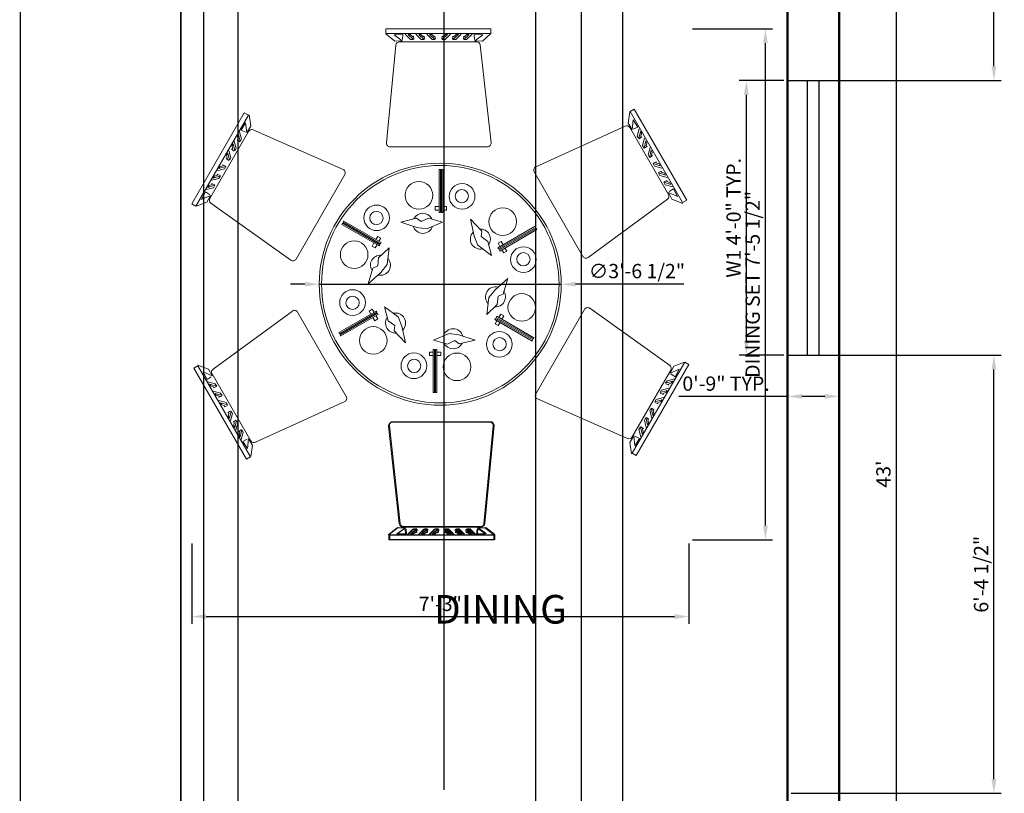
# Model space of a CAD drawing. Units: inches. Extents: x 1905 to 2315, y 3232 to 3824.
# Tile 5 of 8: x 2143 to 2315, y 3479 to 3615. Entities that reach past the tile are written whole.
import ezdxf

# ---------------------------------------------------------------- set-up
doc = ezdxf.new("R2010")
doc.units = ezdxf.units.IN
for name, color, linetype, lineweight in [('A-ANNO-DIMS', 2, 'Continuous', 18), ('A-AREA-IDEN', 7, 'Continuous', 25), ('A-FURN', 8, 'Continuous', 18), ('wall', 2, 'Continuous', 50), ('WINDOW', 60, 'Continuous', 25)]:
    doc.layers.add(name, color=color, linetype=linetype, lineweight=lineweight)
doc.styles.get("Standard").update_dxf_attribs({"font": 'arial.ttf'})
doc.dimstyles.new('ISO-25', dxfattribs={"dimtxt": 2.5, "dimasz": 2.5, "dimexe": 1.25, "dimexo": 0.625, "dimtad": 1, "dimdec": 1, "dimlunit": 3, "dimtxsty": 'Standard', "dimcen": 2.5, "dimadec": 0, "dimazin": 0, "dimtfac": 1, "dimtdec": 1, "dimtmove": 0, "dimatfit": 3, "dimfxl": 1, "dimarcsym": 0})

# ---------------------------------------------------------------- blocks, each defined once
blk = doc.blocks.new('A$C45501D90')
for p, q in [((-242.2, 1133.5), (224, 1133.5)), ((-242.2, 1112.8), (-242.2, 1133.5)), ((224, 1112.8), (-242.2, 1112.8)), ((-242.2, 1111.2), (-202.3, 1079.2)), ((-203.9, 1106.4), (-165.6, 1108)), ((-168.8, 1080.8), (-203.9, 1106.4)), ((-165.6, 1108), (-167.2, 1085.6)), ((-156, 1109.6), (-132, 1085.6)), ((-119.3, 1085.6), (-143.2, 1108)), ((-143.2, 1108), (-133.6, 1108)), ((-133.6, 1108), (-122.5, 1098.4)), ((-122.5, 1098.4), (-119.3, 1101.6)), ((-119.3, 1101.6), (-117.7, 1087.2)), ((-108.1, 1109.6), (-84.1, 1085.6)), ((-71.4, 1085.6), (-95.3, 1108)), ((-95.3, 1108), (-85.7, 1108)), ((-85.7, 1108), (-74.6, 1098.4)), ((-74.6, 1098.4), (-71.4, 1101.6)), ((-71.4, 1101.6), (-69.8, 1087.2)), ((-60.2, 1109.6), (-36.2, 1085.6)), ((-23.5, 1085.6), (-47.4, 1108)), ((-47.4, 1108), (-37.8, 1108)), ((-37.8, 1108), (-26.7, 1098.4)), ((-26.7, 1098.4), (-23.5, 1101.6)), ((-23.5, 1101.6), (-21.9, 1087.2)), ((8.5, 1101.6), (6.9, 1087.2)), ((8.5, 1085.6), (32.4, 1108)), ((11.6, 1098.4), (8.5, 1101.6)), ((22.8, 1108), (11.6, 1098.4)), ((45.2, 1109.6), (21.2, 1085.6)), ((32.4, 1108), (22.8, 1108)), ((56.3, 1101.6), (54.8, 1087.2)), ((56.3, 1085.6), (80.3, 1108)), ((59.5, 1098.4), (56.3, 1101.6)), ((70.7, 1108), (59.5, 1098.4)), ((93.1, 1109.6), (69.1, 1085.6)), ((80.3, 1108), (70.7, 1108)), ((104.2, 1101.6), (102.6, 1087.2)), ((104.2, 1085.6), (128.2, 1108)), ((107.4, 1098.4), (104.2, 1101.6)), ((118.6, 1108), (107.4, 1098.4)), ((141, 1109.6), (117, 1085.6)), ((128.2, 1108), (118.6, 1108)), ((188.9, 1106.4), (150.5, 1108)), ((150.5, 1108), (152.1, 1085.6)), ((153.7, 1080.8), (188.9, 1106.4)), ((224, 1112.8), (187.3, 1079.2)), ((224, 1133.5), (224, 1112.8)), ((-197.3, 1061.6), (-238.9, 627.6)), ((-202.3, 1079.2), (-168.8, 1080.8)), ((161.8, 1076.1), (-181.4, 1076.1)), ((-132, 1085.6), (-119.3, 1085.6)), ((-84.1, 1085.6), (-71.4, 1085.6)), ((-36.2, 1085.6), (-23.5, 1085.6)), ((21.2, 1085.6), (8.5, 1085.6)), ((69.1, 1085.6), (56.3, 1085.6)), ((117, 1085.6), (104.2, 1085.6)), ((187.3, 1079.2), (153.7, 1080.8)), ((225.2, 627.8), (177.6, 1061.8)), ((-1102.7, 357), (-869.7, 760.7)), ((-851.7, 750.4), (-1084.8, 346.6)), ((-869.7, 760.7), (-851.7, 750.4)), ((-848.7, 752.3), (-841, 701.8)), ((841.2, 765.3), (833.5, 714.8)), ((842.6, 766.1), (860.5, 776.5)), ((1075.7, 362.4), (842.6, 766.1)), ((860.5, 776.5), (1093.6, 372.8)), ((-863.7, 716.7), (-884.3, 684.4)), ((-859.2, 673.6), (-863.7, 716.7)), ((-841, 701.8), (-859.2, 673.6)), ((820.7, 701.7), (424.1, 520.7)), ((833.5, 714.8), (851.7, 686.6)), ((851.7, 686.6), (856.2, 729.8)), ((856.2, 729.8), (876.7, 697.4)), ((-851, 678.1), (-1022.6, 380.9)), ((-895.4, 665), (-900.2, 656.7)), ((-900.2, 656.7), (-897.5, 642.2)), ((-888.1, 633.1), (-895.4, 665)), ((-890.4, 676.9), (-881.7, 644.2)), ((-884.3, 684.4), (-864.1, 674.6)), ((-431.1, 509), (-830.8, 684.8)), ((1012.8, 397.9), (841.2, 695.1)), ((876.7, 697.4), (856.6, 687.6)), ((882.9, 689.9), (874.2, 657.2)), ((874.2, 657.2), (880.6, 646.1)), ((880.6, 646.1), (887.9, 678)), ((887.9, 678), (892.7, 669.7)), ((892.7, 669.7), (890, 655.2)), ((-919.4, 623.5), (-924.2, 615.2)), ((-924.2, 615.2), (-921.5, 600.8)), ((-912, 591.6), (-919.4, 623.5)), ((-914.4, 635.4), (-905.6, 602.7)), ((-897.5, 642.2), (-901.9, 641.1)), ((-901.9, 641.1), (-890.2, 632.5)), ((-881.7, 644.2), (-888.1, 633.1)), ((894.4, 654.1), (882.7, 645.5)), ((890, 655.2), (894.4, 654.1)), ((906.9, 648.4), (898.1, 615.7)), ((898.1, 615.7), (904.5, 604.6)), ((904.5, 604.6), (911.9, 636.5)), ((918.3, 612.6), (906.7, 604)), ((911.9, 636.5), (916.7, 628.2)), ((916.7, 628.2), (914, 613.8)), ((914, 613.8), (918.3, 612.6)), ((-943.3, 582), (-948.1, 573.8)), ((-948.1, 573.8), (-945.4, 559.3)), ((-936, 550.1), (-943.3, 582)), ((-938.3, 593.9), (-929.6, 561.2)), ((-921.5, 600.8), (-925.8, 599.6)), ((-925.8, 599.6), (-914.2, 591)), ((-905.6, 602.7), (-912, 591.6)), ((-223, 610.1), (209.4, 610.1)), ((930.8, 606.9), (922.1, 574.2)), ((922.1, 574.2), (928.4, 563.1)), ((928.4, 563.1), (935.8, 595.1)), ((942.3, 571.1), (930.6, 562.6)), ((935.8, 595.1), (940.6, 586.8)), ((940.6, 586.8), (937.9, 572.3)), ((937.9, 572.3), (942.3, 571.1)), ((-978.5, 521.2), (-964.6, 526.1)), ((-964.6, 526.1), (-965.7, 530.5)), ((-965.7, 530.5), (-952.5, 524.7)), ((-945.4, 559.3), (-949.8, 558.1)), ((-949.8, 558.1), (-938.1, 549.6)), ((-929.6, 561.2), (-936, 550.1)), ((950.8, 524.4), (944.4, 535.5)), ((944.4, 535.5), (975.7, 525.9)), ((958.2, 543.5), (945, 537.7)), ((983.5, 515.7), (950.8, 524.4)), ((957.1, 539.1), (958.2, 543.5)), ((970.9, 534.2), (957.1, 539.1)), ((975.7, 525.9), (970.9, 534.2)), ((-975.9, 481), (-1007.2, 471.4)), ((-1002.4, 479.7), (-988.5, 484.6)), ((-991, 502.7), (-958.3, 511.4)), ((-988.5, 484.6), (-989.7, 489)), ((-989.7, 489), (-976.5, 483.2)), ((-951.9, 522.5), (-983.2, 512.9)), ((-983.2, 512.9), (-978.5, 521.2)), ((-982.3, 469.9), (-975.9, 481)), ((-958.3, 511.4), (-951.9, 522.5)), ((-639.9, 111.9), (-423.7, 486.4)), ((-5.6, 508.7, 90.8), (0.4, 508.7, 90.8)), ((-5.6, 317.7, 90.8), (-5.6, 508.7, 90.8)), ((0.4, 508.7, 90.8), (0.4, 317.7, 90.8)), ((5.8, 317.7, 90.8), (5.8, 508.7, 90.8)), ((5.8, 508.7, 90.8), (11.8, 508.7, 90.8)), ((11.8, 508.7, 90.8), (11.8, 317.7, 90.8)), ((416.9, 498.2), (633.1, 123.7)), ((968.4, 494), (999.7, 484.4)), ((974.7, 483), (968.4, 494)), ((982.2, 502), (968.9, 496.2)), ((1007.4, 474.2), (974.7, 483)), ((981, 497.6), (982.2, 502)), ((994.9, 492.7), (981, 497.6)), ((999.7, 484.4), (994.9, 492.7)), ((-999.8, 439.5), (-1031.1, 430)), ((-1031.1, 430), (-1026.3, 438.3)), ((-1026.3, 438.3), (-1012.5, 443.1)), ((-1015, 461.2), (-982.3, 469.9)), ((-1012.5, 443.1), (-1013.6, 447.5)), ((-1013.6, 447.5), (-1000.4, 441.7)), ((-1007.2, 471.4), (-1002.4, 479.7)), ((-1006.2, 428.5), (-999.8, 439.5)), ((998.7, 441.5), (992.3, 452.5)), ((992.3, 452.5), (1023.6, 443)), ((1006.1, 460.5), (992.9, 454.7)), ((1031.4, 432.7), (998.7, 441.5)), ((1005, 456.2), (1006.1, 460.5)), ((1018.8, 451.3), (1005, 456.2)), ((1023.6, 443), (1018.8, 451.3)), ((-1060.1, 376.6), (-1042.3, 410.6)), ((-1020.4, 394.3), (-1060.1, 376.6)), ((-1042.3, 410.6), (-1023.8, 398.1)), ((-1038.9, 419.7), (-1006.2, 428.5)), ((-1035.8, 364.4), (-1020.4, 394.3)), ((1028.3, 377.5), (1012.9, 407.3)), ((1012.9, 407.3), (1052.6, 389.6)), ((1034.8, 423.6), (1016.3, 411.1)), ((1052.6, 389.6), (1034.8, 423.6)), ((-1084.8, 346.6), (-1102.7, 357)), ((-1083.4, 345.8), (-1035.8, 364.4)), ((-1018, 360), (-663, 106.9)), ((656.3, 118.9), (1008.4, 377.1)), ((1075.9, 358.8), (1028.3, 377.5)), ((1093.6, 372.8), (1075.7, 362.4)), ((-22.3, 329.1, 90.8), (-22.3, 344.6, 90.8)), ((-22.3, 344.6, 90.8), (-5.6, 344.6, 90.8)), ((-5.6, 329.1, 90.8), (-22.3, 329.1, 90.8)), ((0.4, 317.7, 90.8), (-5.6, 317.7, 90.8)), ((0.4, 344.6, 90.8), (5.8, 344.6, 90.8)), ((5.8, 329.1, 90.8), (0.4, 329.1, 90.8)), ((11.8, 317.7, 90.8), (5.8, 317.7, 90.8)), ((11.8, 344.6, 90.8), (27.3, 344.6, 90.8)), ((27.3, 329.1, 90.8), (11.8, 329.1, 90.8)), ((27.3, 344.6, 90.8), (27.3, 329.1, 90.8)), ((-436.3, 265.3, 90.8), (-433.3, 270.5, 90.8)), ((-270.9, 169.9, 90.8), (-436.3, 265.3, 90.8)), ((-433.3, 270.5, 90.8), (-267.9, 175, 90.8)), ((-430.6, 275.2, 90.8), (-427.6, 280.3, 90.8)), ((-265.2, 179.7, 90.8), (-430.6, 275.2, 90.8)), ((-427.6, 280.3, 90.8), (-262.3, 184.9, 90.8)), ((-175.3, 276.1, 90.8), (-104.8, 293.2, 90.8)), ((-103.3, 252.4, 90.8), (-175.3, 276.1, 90.8)), ((-104.8, 293.2, 90.8), (-85.5, 278.4, 90.8)), ((-85.5, 278.4, 90.8), (-52.1, 293.9, 90.8)), ((9.5, 276.1, 90.8), (-59.5, 246.5, 90.8)), ((-52.1, 293.9, 90.8), (9.5, 276.1, 90.8)), ((134.3, 288, 90.8), (184.3, 235.5, 90.8)), ((149.7, 213.9, 90.8), (134.3, 288, 90.8)), ((-59.5, 246.5, 90.8), (-103.3, 252.4, 90.8)), ((184.3, 235.5, 90.8), (181.1, 211.4, 90.8)), ((255.2, 161.9, 90.8), (420.6, 257.3, 90.8)), ((423.5, 252.2, 90.8), (258.2, 156.7, 90.8)), ((260.9, 152, 90.8), (426.2, 247.5, 90.8)), ((429.2, 242.3, 90.8), (263.8, 146.9, 90.8)), ((420.6, 257.3, 90.8), (423.5, 252.2, 90.8)), ((426.2, 247.5, 90.8), (429.2, 242.3, 90.8)), ((-302.5, 168.8, 90.8), (-294.2, 183.3, 90.8)), ((-291.2, 188.5, 90.8), (-288.5, 193.1, 90.8)), ((-280.7, 175.5, 90.8), (-289.1, 161.1, 90.8)), ((-285.5, 198.3, 90.8), (-277.8, 211.7, 90.8)), ((-277.8, 211.7, 90.8), (-264.3, 204, 90.8)), ((-275.1, 185.4, 90.8), (-277.8, 180.7, 90.8)), ((-264.3, 204, 90.8), (-272.1, 190.5, 90.8)), ((-267.9, 175, 90.8), (-270.9, 169.9, 90.8)), ((-262.3, 184.9, 90.8), (-265.2, 179.7, 90.8)), ((166.5, 173, 90.8), (149.7, 213.9, 90.8)), ((181.1, 211.4, 90.8), (211.3, 190.3, 90.8)), ((211.3, 190.3, 90.8), (226.7, 128.1, 90.8)), ((256.6, 182, 90.8), (270.1, 189.8, 90.8)), ((265, 167.5, 90.8), (256.6, 182, 90.8)), ((270.1, 189.8, 90.8), (278.4, 175.3, 90.8)), ((-289.1, 161.1, 90.8), (-302.5, 168.8, 90.8)), ((-273.6, 117.6, 90.8), (-227.4, 162.1, 90.8)), ((-227.4, 162.1, 90.8), (-236.2, 87.5, 90.8)), ((226.7, 128.1, 90.8), (166.5, 173, 90.8)), ((258.2, 156.7, 90.8), (255.2, 161.9, 90.8)), ((263.8, 146.9, 90.8), (260.9, 152, 90.8)), ((270.7, 157.7, 90.8), (268, 162.4, 90.8)), ((281.4, 139.1, 90.8), (273.7, 152.5, 90.8)), ((281.4, 170.1, 90.8), (284.1, 165.5, 90.8)), ((294.9, 146.8, 90.8), (281.4, 139.1, 90.8)), ((287.1, 160.3, 90.8), (294.9, 146.8, 90.8)), ((-276.8, 80.9, 90.8), (-273.6, 117.6, 90.8)), ((-236.2, 87.5, 90.8), (-263.2, 52.5, 90.8)), ((-319.8, 2.1, 90.8), (-299.3, 71.7, 90.8)), ((-263.2, 52.5, 90.8), (-319.8, 2.1, 90.8)), ((-299.3, 71.7, 90.8), (-276.8, 80.9, 90.8)), ((242.9, -24.6, 90.8), (299.4, 25.9, 90.8)), ((299.4, 25.9, 90.8), (278.9, -43.7, 90.8)), ((215.8, -59.5, 90.8), (242.9, -24.6, 90.8)), ((278.9, -43.7, 90.8), (256.4, -53, 90.8)), ((207, -134.1, 90.8), (215.8, -59.5, 90.8)), ((256.4, -53, 90.8), (253.2, -89.7, 90.8)), ((-656.3, -118.9), (-1008.4, -377.1)), ((-416.9, -498.2), (-633.1, -123.7)), ((-449.6, -214.4, 90.8), (-284.2, -118.9, 90.8)), ((-281.2, -124.1, 90.8), (-446.6, -219.5, 90.8)), ((-443.9, -224.2, 90.8), (-278.5, -128.7, 90.8)), ((-315.2, -118.9, 90.8), (-301.8, -111.1, 90.8)), ((-307.5, -132.3, 90.8), (-315.2, -118.9, 90.8)), ((-301.8, -111.1, 90.8), (-294, -124.6, 90.8)), ((-291, -129.7, 90.8), (-288.3, -134.4, 90.8)), ((-284.2, -118.9, 90.8), (-281.2, -124.1, 90.8)), ((-278.5, -128.7, 90.8), (-275.5, -133.9, 90.8)), ((-247, -100.1, 90.8), (-186.8, -145, 90.8)), ((-231.7, -162.3, 90.8), (-247, -100.1, 90.8)), ((253.2, -89.7, 90.8), (207, -134.1, 90.8)), ((639.9, -111.9), (423.7, -486.4)), ((1018, -360), (663, -106.9)), ((-275.5, -133.9, 90.8), (-440.9, -229.4, 90.8)), ((-301.8, -142.1, 90.8), (-304.5, -137.5, 90.8)), ((-290.4, -161.8, 90.8), (-298.8, -147.3, 90.8)), ((-277, -154, 90.8), (-290.4, -161.8, 90.8)), ((-285.4, -139.5, 90.8), (-277, -154, 90.8)), ((-201.5, -183.4, 90.8), (-231.7, -162.3, 90.8)), ((-186.8, -145, 90.8), (-170.1, -185.9, 90.8)), ((241.9, -156.9, 90.8), (244.9, -151.7, 90.8)), ((407.3, -252.4, 90.8), (241.9, -156.9, 90.8)), ((244, -176, 90.8), (251.7, -162.5, 90.8)), ((244.9, -151.7, 90.8), (410.3, -247.2, 90.8)), ((247.6, -147.1, 90.8), (250.6, -141.9, 90.8)), ((413, -242.5, 90.8), (247.6, -147.1, 90.8)), ((250.6, -141.9, 90.8), (415.9, -237.4, 90.8)), ((254.7, -157.4, 90.8), (257.4, -152.7, 90.8)), ((265.2, -170.3, 90.8), (257.4, -183.7, 90.8)), ((260.4, -147.6, 90.8), (268.7, -133.1, 90.8)), ((270.8, -160.5, 90.8), (268.1, -165.1, 90.8)), ((268.7, -133.1, 90.8), (282.2, -140.8, 90.8)), ((282.2, -140.8, 90.8), (273.8, -155.3, 90.8)), ((-446.6, -219.5, 90.8), (-449.6, -214.4, 90.8)), ((-204.7, -207.6, 90.8), (-201.5, -183.4, 90.8)), ((-154.7, -260.1, 90.8), (-204.7, -207.6, 90.8)), ((-170.1, -185.9, 90.8), (-154.7, -260.1, 90.8)), ((257.4, -183.7, 90.8), (244, -176, 90.8)), ((-440.9, -229.4, 90.8), (-443.9, -224.2, 90.8)), ((-29.8, -248.2, 90.8), (39.2, -218.5, 90.8)), ((31.8, -266, 90.8), (-29.8, -248.2, 90.8)), ((65.2, -250.4, 90.8), (31.8, -266, 90.8)), ((39.2, -218.5, 90.8), (83, -224.4, 90.8)), ((84.4, -265.2, 90.8), (65.2, -250.4, 90.8)), ((83, -224.4, 90.8), (154.9, -248.2, 90.8)), ((154.9, -248.2, 90.8), (84.4, -265.2, 90.8)), ((410.3, -247.2, 90.8), (407.3, -252.4, 90.8)), ((415.9, -237.4, 90.8), (413, -242.5, 90.8)), ((-47.6, -316.6, 90.8), (-47.6, -301.1, 90.8)), ((-47.6, -301.1, 90.8), (-32.1, -301.1, 90.8)), ((-32.1, -480.7, 90.8), (-32.1, -289.8, 90.8)), ((-32.1, -289.8, 90.8), (-26.1, -289.8, 90.8)), ((-26.1, -289.8, 90.8), (-26.1, -480.7, 90.8)), ((-26.1, -301.1, 90.8), (-20.8, -301.1, 90.8)), ((-20.8, -480.7, 90.8), (-20.8, -289.8, 90.8)), ((-20.8, -289.8, 90.8), (-14.8, -289.8, 90.8)), ((-14.8, -289.8, 90.8), (-14.8, -480.7, 90.8)), ((-14.8, -301.1, 90.8), (1.9, -301.1, 90.8)), ((1.9, -301.1, 90.8), (1.9, -316.6, 90.8)), ((-32.1, -316.6, 90.8), (-47.6, -316.6, 90.8)), ((-20.8, -316.6, 90.8), (-26.1, -316.6, 90.8)), ((1.9, -316.6, 90.8), (-14.8, -316.6, 90.8)), ((851.7, -750.4), (1084.8, -346.6)), ((1083.4, -345.8), (1035.8, -364.4)), ((1084.8, -346.6), (1102.7, -357)), ((-1093.6, -372.8), (-1075.7, -362.4)), ((-860.5, -776.5), (-1093.6, -372.8)), ((-1075.9, -358.8), (-1028.3, -377.5)), ((-1075.7, -362.4), (-842.6, -766.1)), ((-1052.6, -389.6), (-1034.8, -423.6)), ((-1012.9, -407.3), (-1052.6, -389.6)), ((-1028.3, -377.5), (-1012.9, -407.3)), ((851, -678.1), (1022.6, -380.9)), ((1102.7, -357), (869.7, -760.7)), ((1035.8, -364.4), (1020.4, -394.3)), ((1020.4, -394.3), (1060.1, -376.6)), ((1060.1, -376.6), (1042.3, -410.6)), ((-1034.8, -423.6), (-1016.3, -411.1)), ((-1031.4, -432.7), (-998.7, -441.5)), ((-1012.8, -397.9), (-841.2, -695.1)), ((1006.2, -428.5), (999.8, -439.5)), ((999.8, -439.5), (1031.1, -430)), ((1038.9, -419.7), (1006.2, -428.5)), ((1042.3, -410.6), (1023.8, -398.1)), ((1031.1, -430), (1026.3, -438.3)), ((-1023.6, -443), (-1018.8, -451.3)), ((-992.3, -452.5), (-1023.6, -443)), ((-1018.8, -451.3), (-1005, -456.2)), ((-1007.4, -474.2), (-974.7, -483)), ((-1006.1, -460.5), (-992.9, -454.7)), ((-1005, -456.2), (-1006.1, -460.5)), ((-998.7, -441.5), (-992.3, -452.5)), ((982.3, -469.9), (975.9, -481)), ((975.9, -481), (1007.2, -471.4)), ((1015, -461.2), (982.3, -469.9)), ((1002.4, -479.7), (988.5, -484.6)), ((1013.6, -447.5), (1000.4, -441.7)), ((1007.2, -471.4), (1002.4, -479.7)), ((1026.3, -438.3), (1012.5, -443.1)), ((1012.5, -443.1), (1013.6, -447.5)), ((-968.4, -494), (-999.7, -484.4)), ((-999.7, -484.4), (-994.9, -492.7)), ((-994.9, -492.7), (-981, -497.6)), ((-983.5, -515.7), (-950.8, -524.4)), ((-982.2, -502), (-968.9, -496.2)), ((-981, -497.6), (-982.2, -502)), ((-974.7, -483), (-968.4, -494)), ((-820.7, -701.7), (-424.1, -520.7)), ((-26.1, -480.7, 90.8), (-32.1, -480.7, 90.8)), ((-14.8, -480.7, 90.8), (-20.8, -480.7, 90.8)), ((431.1, -509), (830.8, -684.8)), ((958.3, -511.4), (951.9, -522.5)), ((951.9, -522.5), (983.2, -512.9)), ((991, -502.7), (958.3, -511.4)), ((978.5, -521.2), (964.6, -526.1)), ((989.7, -489), (976.5, -483.2)), ((983.2, -512.9), (978.5, -521.2)), ((988.5, -484.6), (989.7, -489)), ((-944.4, -535.5), (-975.7, -525.9)), ((-975.7, -525.9), (-970.9, -534.2)), ((-970.9, -534.2), (-957.1, -539.1)), ((-958.2, -543.5), (-945, -537.7)), ((-957.1, -539.1), (-958.2, -543.5)), ((-950.8, -524.4), (-944.4, -535.5)), ((-942.3, -571.1), (-930.6, -562.6)), ((-928.4, -563.1), (-935.8, -595.1)), ((-922.1, -574.2), (-928.4, -563.1)), ((929.6, -561.2), (936, -550.1)), ((938.3, -593.9), (929.6, -561.2)), ((936, -550.1), (943.3, -582)), ((949.8, -558.1), (938.1, -549.6)), ((945.4, -559.3), (949.8, -558.1)), ((948.1, -573.8), (945.4, -559.3)), ((965.7, -530.5), (952.5, -524.7)), ((964.6, -526.1), (965.7, -530.5)), ((-937.9, -572.3), (-942.3, -571.1)), ((-940.6, -586.8), (-937.9, -572.3)), ((-935.8, -595.1), (-940.6, -586.8)), ((-930.8, -606.9), (-922.1, -574.2)), ((-918.3, -612.6), (-906.7, -604)), ((-904.5, -604.6), (-911.9, -636.5)), ((-898.1, -615.7), (-904.5, -604.6)), ((218.9, -611.6), (-213.5, -611.6)), ((223, -610.1), (-209.4, -610.1)), ((905.6, -602.7), (912, -591.6)), ((914.4, -635.4), (905.6, -602.7)), ((912, -591.6), (919.4, -623.5)), ((925.8, -599.6), (914.2, -591)), ((921.5, -600.8), (925.8, -599.6)), ((924.2, -615.2), (921.5, -600.8)), ((943.3, -582), (948.1, -573.8)), ((-914, -613.8), (-918.3, -612.6)), ((-916.7, -628.2), (-914, -613.8)), ((-911.9, -636.5), (-916.7, -628.2)), ((-906.9, -648.4), (-898.1, -615.7)), ((-894.4, -654.1), (-882.7, -645.5)), ((-890, -655.2), (-894.4, -654.1)), ((-892.7, -669.7), (-890, -655.2)), ((-880.6, -646.1), (-887.9, -678)), ((-874.2, -657.2), (-880.6, -646.1)), ((-229.3, -629.3), (-181.8, -1063.3)), ((-225.2, -627.8), (-177.6, -1061.8)), ((193.2, -1063.1), (234.8, -629.1)), ((197.3, -1061.6), (238.9, -627.6)), ((881.7, -644.2), (888.1, -633.1)), ((890.4, -676.9), (881.7, -644.2)), ((888.1, -633.1), (895.4, -665)), ((901.9, -641.1), (890.2, -632.5)), ((897.5, -642.2), (901.9, -641.1)), ((900.2, -656.7), (897.5, -642.2)), ((919.4, -623.5), (924.2, -615.2)), ((-887.9, -678), (-892.7, -669.7)), ((-882.9, -689.9), (-874.2, -657.2)), ((-876.7, -697.4), (-856.6, -687.6)), ((-856.2, -729.8), (-876.7, -697.4)), ((-851.7, -686.6), (-856.2, -729.8)), ((-833.5, -714.8), (-851.7, -686.6)), ((841, -701.8), (859.2, -673.6)), ((859.2, -673.6), (863.7, -716.7)), ((863.7, -716.7), (884.3, -684.4)), ((884.3, -684.4), (864.1, -674.6)), ((895.4, -665), (900.2, -656.7)), ((-841.2, -765.3), (-833.5, -714.8)), ((848.7, -752.3), (841, -701.8)), ((-842.6, -766.1), (-860.5, -776.5)), ((869.7, -760.7), (851.7, -750.4)), ((-231.3, -1112.7), (-191.4, -1080.8)), ((-227.2, -1111.2), (-187.3, -1079.2)), ((-157.9, -1082.4), (-193, -1107.9)), ((-191.4, -1080.8), (-157.9, -1082.4)), ((-153.7, -1080.8), (-188.9, -1106.4)), ((-187.3, -1079.2), (-153.7, -1080.8)), ((-165.9, -1077.6), (177.3, -1077.6)), ((-161.8, -1076.1), (181.4, -1076.1)), ((-154.7, -1109.5), (-156.3, -1087.1)), ((-150.5, -1108), (-152.1, -1085.6)), ((-145.1, -1111.1), (-121.1, -1087.1)), ((-141, -1109.6), (-117, -1085.6)), ((-108.4, -1087.1), (-132.3, -1109.5)), ((-104.2, -1085.6), (-128.2, -1108)), ((-121.1, -1087.1), (-108.4, -1087.1)), ((-117, -1085.6), (-104.2, -1085.6)), ((-108.4, -1103.1), (-106.8, -1088.7)), ((-104.2, -1101.6), (-102.6, -1087.2)), ((-97.2, -1111.1), (-73.2, -1087.1)), ((-93.1, -1109.6), (-69.1, -1085.6)), ((-60.5, -1087.1), (-84.4, -1109.5)), ((-56.3, -1085.6), (-80.3, -1108)), ((-73.2, -1087.1), (-60.5, -1087.1)), ((-69.1, -1085.6), (-56.3, -1085.6)), ((-60.5, -1103.1), (-58.9, -1088.7)), ((-56.3, -1101.6), (-54.8, -1087.2)), ((-49.3, -1111.1), (-25.3, -1087.1)), ((-45.2, -1109.6), (-21.2, -1085.6)), ((-12.6, -1087.1), (-36.5, -1109.5)), ((-8.5, -1085.6), (-32.4, -1108)), ((-25.3, -1087.1), (-12.6, -1087.1)), ((-21.2, -1085.6), (-8.5, -1085.6)), ((-12.6, -1103.1), (-11, -1088.7)), ((-8.5, -1101.6), (-6.9, -1087.2)), ((19.4, -1103.1), (17.8, -1088.7)), ((19.4, -1087.1), (43.3, -1109.5)), ((32.1, -1087.1), (19.4, -1087.1)), ((23.5, -1101.6), (21.9, -1087.2)), ((23.5, -1085.6), (47.4, -1108)), ((36.2, -1085.6), (23.5, -1085.6)), ((56.1, -1111.1), (32.1, -1087.1)), ((60.2, -1109.6), (36.2, -1085.6)), ((67.3, -1103.1), (65.7, -1088.7)), ((67.3, -1087.1), (91.2, -1109.5)), ((80, -1087.1), (67.3, -1087.1)), ((71.4, -1101.6), (69.8, -1087.2)), ((71.4, -1085.6), (95.3, -1108)), ((84.1, -1085.6), (71.4, -1085.6)), ((104, -1111.1), (80, -1087.1)), ((108.1, -1109.6), (84.1, -1085.6)), ((115.1, -1103.1), (113.6, -1088.7)), ((115.1, -1087.1), (139.1, -1109.5)), ((127.9, -1087.1), (115.1, -1087.1)), ((119.3, -1101.6), (117.7, -1087.2)), ((119.3, -1085.6), (143.2, -1108)), ((132, -1085.6), (119.3, -1085.6)), ((151.9, -1111.1), (127.9, -1087.1)), ((156, -1109.6), (132, -1085.6)), ((161.4, -1109.5), (163, -1087.1)), ((198.2, -1080.8), (164.6, -1082.4)), ((164.6, -1082.4), (199.8, -1107.9)), ((165.6, -1108), (167.2, -1085.6)), ((202.3, -1079.2), (168.8, -1080.8)), ((168.8, -1080.8), (203.9, -1106.4)), ((238.1, -1112.7), (198.2, -1080.8)), ((242.2, -1111.2), (202.3, -1079.2)), ((-228.1, -1114.3), (238.1, -1114.3)), ((-228.1, -1135), (-228.1, -1114.3)), ((238.1, -1135), (-228.1, -1135)), ((-224, -1112.8), (242.2, -1112.8)), ((-224, -1133.5), (-224, -1112.8)), ((242.2, -1133.5), (-224, -1133.5)), ((-193, -1107.9), (-154.7, -1109.5)), ((-188.9, -1106.4), (-150.5, -1108)), ((-132.3, -1109.5), (-122.7, -1109.5)), ((-128.2, -1108), (-118.6, -1108)), ((-122.7, -1109.5), (-111.6, -1099.9)), ((-118.6, -1108), (-107.4, -1098.4)), ((-111.6, -1099.9), (-108.4, -1103.1)), ((-107.4, -1098.4), (-104.2, -1101.6)), ((-84.4, -1109.5), (-74.8, -1109.5)), ((-80.3, -1108), (-70.7, -1108)), ((-74.8, -1109.5), (-63.7, -1099.9)), ((-70.7, -1108), (-59.5, -1098.4)), ((-63.7, -1099.9), (-60.5, -1103.1)), ((-59.5, -1098.4), (-56.3, -1101.6)), ((-36.5, -1109.5), (-26.9, -1109.5)), ((-32.4, -1108), (-22.8, -1108)), ((-26.9, -1109.5), (-15.8, -1099.9)), ((-22.8, -1108), (-11.6, -1098.4)), ((-15.8, -1099.9), (-12.6, -1103.1)), ((-11.6, -1098.4), (-8.5, -1101.6)), ((22.6, -1099.9), (19.4, -1103.1)), ((33.7, -1109.5), (22.6, -1099.9)), ((26.7, -1098.4), (23.5, -1101.6)), ((37.8, -1108), (26.7, -1098.4)), ((43.3, -1109.5), (33.7, -1109.5)), ((47.4, -1108), (37.8, -1108)), ((70.4, -1099.9), (67.3, -1103.1)), ((81.6, -1109.5), (70.4, -1099.9)), ((74.6, -1098.4), (71.4, -1101.6)), ((85.7, -1108), (74.6, -1098.4)), ((91.2, -1109.5), (81.6, -1109.5)), ((95.3, -1108), (85.7, -1108)), ((118.3, -1099.9), (115.1, -1103.1)), ((129.5, -1109.5), (118.3, -1099.9)), ((122.5, -1098.4), (119.3, -1101.6)), ((133.6, -1108), (122.5, -1098.4)), ((139.1, -1109.5), (129.5, -1109.5)), ((143.2, -1108), (133.6, -1108)), ((199.8, -1107.9), (161.4, -1109.5)), ((203.9, -1106.4), (165.6, -1108)), ((238.1, -1114.3), (238.1, -1135)), ((242.2, -1112.8), (242.2, -1133.5))]:
    blk.add_line(p, q)
for centre, radius in [((0, 0), 537), ((0, 0), 527), ((-94.8, 394.7, 90.8), 61.3), ((96.9, 390, 90.8), 56.9), ((95.5, 390.7, 90.8), 29.4), ((-282.3, 294.7, 90.8), 56.9), ((-283.5, 293.9, 90.8), 29.4), ((277.2, 277.6, 90.8), 61.3), ((-382.1, 131.1, 90.8), 61.3), ((369, 109.3, 90.8), 56.9), ((368.9, 110.8, 90.8), 29.4), ((-389.3, -81.3, 90.8), 56.9), ((361.8, -103.1, 90.8), 61.3), ((-389.2, -82.8, 90.8), 29.4), ((-297.5, -249.6, 90.8), 61.3), ((261.9, -266.7, 90.8), 56.9), ((263.2, -265.9, 90.8), 29.4), ((-117.2, -362, 90.8), 56.9), ((74.4, -366.7, 90.8), 61.3), ((-115.9, -362.7, 90.8), 29.4)]:
    blk.add_circle(centre, radius)
for centre, radius, start, end in [((-181.4, 1060.1), 16, 90, 174.5199), ((161.8, 1060.1), 16, 6.2572, 90), ((827.4, 687.1), 16, 30, 114.5199), ((-837.2, 670.1), 16, 66.2572, 150), ((-223, 626.1), 16, 174.5199, 270), ((209.4, 626.1), 16, 270, 6.2572), ((-437.5, 494.4), 16, 330, 66.2572), ((430.7, 506.2), 16, 114.5199, 210), ((999, 389.9), 16, 306.2572, 30), ((-1008.8, 373), 16, 150, 234.5199), ((-77.3, 270.2, 90.8), 44.6, 25.8558, 153.3359), ((-77.3, 270.2, 90.8), 44.6, 195.9338, 342.9389), ((178.1, 200.3, 90.8), 44.6, 135.9338, 282.9389), ((178.1, 200.3, 90.8), 44.6, 325.8558, 93.3359), ((-653.7, 119.9), 16, 234.5199, 330), ((-265.7, 83.9, 90.8), 44.6, 85.8558, 213.3359), ((-265.7, 83.9, 90.8), 44.6, 255.9338, 42.9389), ((646.9, 131.7), 16, 210, 306.2572), ((245.3, -55.9, 90.8), 44.6, 75.9338, 222.9389), ((245.3, -55.9, 90.8), 44.6, 265.8558, 33.3359), ((-646.9, -131.7), 16, 30, 126.2572), ((-198.5, -172.3, 90.8), 44.6, 315.9338, 102.9389), ((653.7, -119.9), 16, 54.5199, 150), ((-198.5, -172.3, 90.8), 44.6, 145.8558, 273.3359), ((57, -242.2, 90.8), 44.6, 15.9338, 162.9389), ((57, -242.2, 90.8), 44.6, 205.8558, 333.3359), ((-999, -389.9), 16, 126.2572, 210), ((1008.8, -373), 16, 330, 54.5199), ((-430.7, -506.2), 16, 294.5199, 30), ((437.5, -494.4), 16, 150, 246.2572), ((-213.5, -627.6), 16, 90, 186.2572), ((-209.4, -626.1), 16, 90, 186.2572), ((218.9, -627.6), 16, 354.5199, 90), ((223, -626.1), 16, 354.5199, 90), ((-827.4, -687.1), 16, 210, 294.5199), ((837.2, -670.1), 16, 246.2572, 330), ((-165.9, -1061.6), 16, 186.2572, 270), ((-161.8, -1060.1), 16, 186.2572, 270), ((177.3, -1061.6), 16, 270, 354.5199), ((181.4, -1060.1), 16, 270, 354.5199)]:
    blk.add_arc(centre, radius, start, end)
blk = doc.blocks.new('*D16')
at = {"layer": 'A-ANNO-DIMS', "color": 0, "lineweight": -2, "transparency": 16777216}
for p, q in [((2286.63, 3793.23), (2297.23, 3793.23)), ((2295.98, 3790.73), (2295.98, 3279.73)), ((2286.63, 3277.23), (2297.23, 3277.23))]:
    blk.add_line(p, q, dxfattribs=at)
at = {"layer": 'A-ANNO-DIMS', "color": 0, "transparency": 16777216}
for points in [[(2295.57, 3790.73), (2296.4, 3790.73), (2295.98, 3793.23)], [(2295.57, 3279.73), (2296.4, 3279.73), (2295.98, 3277.23)]]:
    blk.add_solid(points, dxfattribs=at)
at = {"layer": 'Defpoints', "color": 0, "transparency": 16777216}
for p in [(2286.01, 3793.23), (2286.01, 3277.23), (2295.98, 3277.23)]:
    blk.add_point(p, dxfattribs=at)
at = {"layer": 'A-ANNO-DIMS', "color": 0, "transparency": 16777216, "insert": (2294.08, 3535.23), "char_height": 2.5, "attachment_point": 5, "rotation": 90}
blk.add_mtext("43'", dxfattribs=at)
blk = doc.blocks.new('WIN-48IN')
for p, q in [((0, 9), (0, 0)), ((0, 9), (48, 9)), ((48, 9), (48, 0)), ((0, 5.5), (48, 5.5)), ((0, 3.5), (48, 3.5)), ((0, 0), (48, 0))]:
    blk.add_line(p, q)
blk = doc.blocks.new('*D21')
at = {"layer": 'A-ANNO-DIMS', "color": 0, "lineweight": -2, "transparency": 16777216}
for p, q in [((2276.38, 3604.01), (2268.56, 3604.01)), ((2269.81, 3558.51), (2269.81, 3601.51)), ((2276.38, 3556.01), (2268.56, 3556.01))]:
    blk.add_line(p, q, dxfattribs=at)
at = {"layer": 'A-ANNO-DIMS', "color": 0, "transparency": 16777216}
for points in [[(2269.39, 3601.51), (2270.22, 3601.51), (2269.81, 3604.01)], [(2269.39, 3558.51), (2270.22, 3558.51), (2269.81, 3556.01)]]:
    blk.add_solid(points, dxfattribs=at)
at = {"layer": 'Defpoints', "color": 0, "transparency": 16777216}
for p in [(2269.81, 3604.01), (2277.01, 3604.01), (2277.01, 3556.01)]:
    blk.add_point(p, dxfattribs=at)
at = {"layer": 'A-ANNO-DIMS', "color": 0, "transparency": 16777216, "insert": (2267.91, 3580.01), "char_height": 2.5, "attachment_point": 5, "rotation": 90}
blk.add_mtext('W1 4\'-0" TYP.', dxfattribs=at)
blk = doc.blocks.new('*D22')
at = {"layer": 'A-ANNO-DIMS', "color": 0, "lineweight": -2, "transparency": 16777216}
for p, q in [((2277.01, 3555.38), (2277.01, 3547.56)), ((2286.01, 3555.38), (2286.01, 3547.56)), ((2277.01, 3548.81), (2258.02, 3548.81)), ((2283.51, 3548.81), (2279.51, 3548.81))]:
    blk.add_line(p, q, dxfattribs=at)
at = {"layer": 'A-ANNO-DIMS', "color": 0, "transparency": 16777216}
for points in [[(2279.51, 3549.22), (2279.51, 3548.39), (2277.01, 3548.81)], [(2283.51, 3549.22), (2283.51, 3548.39), (2286.01, 3548.81)]]:
    blk.add_solid(points, dxfattribs=at)
at = {"layer": 'Defpoints', "color": 0, "transparency": 16777216}
for p in [(2277.01, 3556.01), (2286.01, 3556.01), (2277.01, 3548.81)]:
    blk.add_point(p, dxfattribs=at)
at = {"layer": 'A-ANNO-DIMS', "color": 0, "transparency": 16777216, "insert": (2266.26, 3550.71), "char_height": 2.5, "attachment_point": 5}
blk.add_mtext('0\'-9" TYP.', dxfattribs=at)
blk = doc.blocks.new('*D33')
at = {"layer": 'A-ANNO-DIMS', "color": 0, "lineweight": -2, "transparency": 16777216}
for p, q in [((2260.37, 3613.04), (2274.39, 3613.04)), ((2273.14, 3526.23), (2273.14, 3610.54)), ((2260.37, 3523.73), (2274.39, 3523.73))]:
    blk.add_line(p, q, dxfattribs=at)
at = {"layer": 'A-ANNO-DIMS', "color": 0, "transparency": 16777216}
for points in [[(2272.73, 3610.54), (2273.56, 3610.54), (2273.14, 3613.04)], [(2272.73, 3526.23), (2273.56, 3526.23), (2273.14, 3523.73)]]:
    blk.add_solid(points, dxfattribs=at)
at = {"layer": 'Defpoints', "color": 0, "transparency": 16777216}
for p in [(2259.75, 3613.04), (2273.14, 3613.04), (2259.75, 3523.73)]:
    blk.add_point(p, dxfattribs=at)
at = {"layer": 'A-ANNO-DIMS', "color": 0, "transparency": 16777216, "insert": (2271.23, 3568.38), "char_height": 2.5, "attachment_point": 5, "rotation": 90}
blk.add_mtext('DINING SET 7\'-5 1/2"', dxfattribs=at)
blk = doc.blocks.new('*D34')
at = {"layer": 'A-ANNO-DIMS', "color": 0, "lineweight": -2, "transparency": 16777216}
for p, q in [((2172.92, 3523.1), (2172.92, 3509.08)), ((2259.75, 3523.1), (2259.75, 3509.08)), ((2175.42, 3510.33), (2257.25, 3510.33))]:
    blk.add_line(p, q, dxfattribs=at)
at = {"layer": 'A-ANNO-DIMS', "color": 0, "transparency": 16777216}
for points in [[(2175.42, 3510.75), (2175.42, 3509.91), (2172.92, 3510.33)], [(2257.25, 3510.75), (2257.25, 3509.91), (2259.75, 3510.33)]]:
    blk.add_solid(points, dxfattribs=at)
at = {"layer": 'Defpoints', "color": 0, "transparency": 16777216}
for p in [(2172.92, 3523.73), (2259.75, 3523.73), (2259.75, 3510.33)]:
    blk.add_point(p, dxfattribs=at)
at = {"layer": 'A-ANNO-DIMS', "color": 0, "transparency": 16777216, "insert": (2216.33, 3512.23), "char_height": 2.5, "attachment_point": 5}
blk.add_mtext('7\'-3"', dxfattribs=at)
blk = doc.blocks.new('*D41')
at = {"layer": 'A-ANNO-DIMS', "color": 0, "lineweight": -2, "transparency": 16777216}
for p, q in [((2095.01, 3663.61), (2095.01, 3232.16)), ((2171.01, 3663.61), (2171.01, 3232.16)), ((2097.51, 3233.41), (2168.51, 3233.41))]:
    blk.add_line(p, q, dxfattribs=at)
at = {"layer": 'A-ANNO-DIMS', "color": 0, "transparency": 16777216}
for points in [[(2097.51, 3233.83), (2097.51, 3233), (2095.01, 3233.41)], [(2168.51, 3233.83), (2168.51, 3233), (2171.01, 3233.41)]]:
    blk.add_solid(points, dxfattribs=at)
at = {"layer": 'Defpoints', "color": 0, "transparency": 16777216}
for p in [(2095.01, 3664.23), (2171.01, 3664.23), (2171.01, 3233.41)]:
    blk.add_point(p, dxfattribs=at)
at = {"layer": 'A-ANNO-DIMS', "color": 0, "transparency": 16777216, "insert": (2133.01, 3235.31), "char_height": 2.5, "attachment_point": 5}
blk.add_mtext('6\'-4"', dxfattribs=at)
blk = doc.blocks.new('*D53')
at = {"layer": 'A-ANNO-DIMS', "color": 0, "lineweight": -2, "transparency": 16777216}
for p, q in [((2277.63, 3556.01), (2314.32, 3556.01)), ((2313.07, 3481.95), (2313.07, 3553.51)), ((2277.63, 3479.45), (2314.32, 3479.45))]:
    blk.add_line(p, q, dxfattribs=at)
at = {"layer": 'A-ANNO-DIMS', "color": 0, "transparency": 16777216}
for points in [[(2312.65, 3553.51), (2313.48, 3553.51), (2313.07, 3556.01)], [(2312.65, 3481.95), (2313.48, 3481.95), (2313.07, 3479.45)]]:
    blk.add_solid(points, dxfattribs=at)
at = {"layer": 'Defpoints', "color": 0, "transparency": 16777216}
for p in [(2277.01, 3556.01), (2313.07, 3556.01), (2277.01, 3479.45)]:
    blk.add_point(p, dxfattribs=at)
at = {"layer": 'A-ANNO-DIMS', "color": 0, "transparency": 16777216, "insert": (2311.15, 3517.73), "char_height": 2.5, "attachment_point": 5, "rotation": 90}
blk.add_mtext('6\'-4 1/2"', dxfattribs=at)
blk = doc.blocks.new('*D54')
at = {"layer": 'A-ANNO-DIMS', "color": 0, "lineweight": -2, "transparency": 16777216}
for p, q in [((2277.63, 3660.23), (2314.32, 3660.23)), ((2313.07, 3606.51), (2313.07, 3657.73)), ((2277.63, 3604.01), (2314.32, 3604.01))]:
    blk.add_line(p, q, dxfattribs=at)
at = {"layer": 'A-ANNO-DIMS', "color": 0, "transparency": 16777216}
for points in [[(2312.65, 3657.73), (2313.48, 3657.73), (2313.07, 3660.23)], [(2312.65, 3606.51), (2313.48, 3606.51), (2313.07, 3604.01)]]:
    blk.add_solid(points, dxfattribs=at)
at = {"layer": 'Defpoints', "color": 0, "transparency": 16777216}
for p in [(2277.01, 3660.23), (2313.07, 3660.23), (2277.01, 3604.01)]:
    blk.add_point(p, dxfattribs=at)
at = {"layer": 'A-ANNO-DIMS', "color": 0, "transparency": 16777216, "insert": (2311.17, 3632.12), "char_height": 2.5, "attachment_point": 5, "rotation": 90}
blk.add_mtext('4\'-8"', dxfattribs=at)
blk = doc.blocks.new('*D62')
at = {"layer": 'A-ANNO-DIMS', "color": 0, "lineweight": -2, "transparency": 16777216}
for p, q in [((2233.01, 3322.86), (2233.01, 3821.54)), ((2241.01, 3322.86), (2241.01, 3821.54)), ((2235.51, 3820.29), (2238.51, 3820.29))]:
    blk.add_line(p, q, dxfattribs=at)
at = {"layer": 'A-ANNO-DIMS', "color": 0, "transparency": 16777216}
for points in [[(2235.51, 3820.71), (2235.51, 3819.88), (2233.01, 3820.29)], [(2238.51, 3820.71), (2238.51, 3819.88), (2241.01, 3820.29)]]:
    blk.add_solid(points, dxfattribs=at)
at = {"layer": 'Defpoints', "color": 0, "transparency": 16777216}
for p in [(2241.01, 3820.29), (2233.01, 3322.23), (2241.01, 3322.23)]:
    blk.add_point(p, dxfattribs=at)
at = {"layer": 'A-ANNO-DIMS', "color": 0, "transparency": 16777216, "insert": (2237.01, 3822.19), "char_height": 2.5, "attachment_point": 5}
blk.add_mtext('0\'-8"', dxfattribs=at)
blk = doc.blocks.new('*D63')
at = {"layer": 'A-ANNO-DIMS', "color": 0, "lineweight": -2, "transparency": 16777216}
for p, q in [((2171.01, 3480.07), (2171.01, 3821.54)), ((2175.01, 3476.07), (2175.01, 3821.54)), ((2168.51, 3820.29), (2166.01, 3820.29)), ((2171.01, 3820.29), (2175.01, 3820.29)), ((2177.51, 3820.29), (2187.9, 3820.29))]:
    blk.add_line(p, q, dxfattribs=at)
at = {"layer": 'A-ANNO-DIMS', "color": 0, "transparency": 16777216}
for points in [[(2168.51, 3820.71), (2168.51, 3819.88), (2171.01, 3820.29)], [(2177.51, 3820.71), (2177.51, 3819.88), (2175.01, 3820.29)]]:
    blk.add_solid(points, dxfattribs=at)
at = {"layer": 'Defpoints', "color": 0, "transparency": 16777216}
for p in [(2175.01, 3820.29), (2171.01, 3479.45), (2175.01, 3475.45)]:
    blk.add_point(p, dxfattribs=at)
at = {"layer": 'A-ANNO-DIMS', "color": 0, "transparency": 16777216, "insert": (2183.96, 3822.19), "char_height": 2.5, "attachment_point": 5}
blk.add_mtext('0\'-4"', dxfattribs=at)
blk = doc.blocks.new('*D66')
at = {"layer": 'A-ANNO-DIMS', "color": 0, "lineweight": -2, "transparency": 16777216}
for p, q in [((2248.2, 3393.73), (2248.2, 3821.54)), ((2277.01, 3383.48), (2277.01, 3821.54)), ((2250.7, 3820.29), (2274.51, 3820.29))]:
    blk.add_line(p, q, dxfattribs=at)
at = {"layer": 'A-ANNO-DIMS', "color": 0, "transparency": 16777216}
for points in [[(2250.7, 3820.71), (2250.7, 3819.88), (2248.2, 3820.29)], [(2274.51, 3820.71), (2274.51, 3819.88), (2277.01, 3820.29)]]:
    blk.add_solid(points, dxfattribs=at)
at = {"layer": 'Defpoints', "color": 0, "transparency": 16777216}
for p in [(2277.01, 3820.29), (2248.2, 3393.11), (2277.01, 3382.85)]:
    blk.add_point(p, dxfattribs=at)
at = {"layer": 'A-ANNO-DIMS', "color": 0, "transparency": 16777216, "insert": (2262.6, 3822.19), "char_height": 2.5, "attachment_point": 5}
blk.add_mtext('2\'-5"', dxfattribs=at)
blk = doc.blocks.new('*D70')
at = {"layer": 'A-ANNO-DIMS', "color": 0, "lineweight": -2, "transparency": 16777216}
for p, q in [((2175.01, 3476.07), (2175.01, 3821.54)), ((2181.01, 3476.07), (2181.01, 3821.54)), ((2172.51, 3820.29), (2170.01, 3820.29)), ((2175.01, 3820.29), (2181.01, 3820.29)), ((2183.51, 3820.29), (2193.9, 3820.29))]:
    blk.add_line(p, q, dxfattribs=at)
at = {"layer": 'A-ANNO-DIMS', "color": 0, "transparency": 16777216}
for points in [[(2172.51, 3820.71), (2172.51, 3819.88), (2175.01, 3820.29)], [(2183.51, 3820.71), (2183.51, 3819.88), (2181.01, 3820.29)]]:
    blk.add_solid(points, dxfattribs=at)
at = {"layer": 'Defpoints', "color": 0, "transparency": 16777216}
for p in [(2181.01, 3820.29), (2175.01, 3475.45), (2181.01, 3475.45)]:
    blk.add_point(p, dxfattribs=at)
at = {"layer": 'A-ANNO-DIMS', "color": 0, "transparency": 16777216, "insert": (2189.96, 3822.19), "char_height": 2.5, "attachment_point": 5}
blk.add_mtext('0\'-6"', dxfattribs=at)
blk = doc.blocks.new('*D71')
at = {"layer": 'A-ANNO-DIMS', "color": 0, "lineweight": -2, "transparency": 16777216}
for p, q in [((2217.01, 3480.07), (2217.01, 3821.54)), ((2277.01, 3476.07), (2277.01, 3821.54)), ((2219.51, 3820.29), (2274.51, 3820.29))]:
    blk.add_line(p, q, dxfattribs=at)
at = {"layer": 'A-ANNO-DIMS', "color": 0, "transparency": 16777216}
for points in [[(2219.51, 3820.71), (2219.51, 3819.88), (2217.01, 3820.29)], [(2274.51, 3820.71), (2274.51, 3819.88), (2277.01, 3820.29)]]:
    blk.add_solid(points, dxfattribs=at)
at = {"layer": 'Defpoints', "color": 0, "transparency": 16777216}
for p in [(2277.01, 3820.29), (2217.01, 3479.45), (2277.01, 3475.45)]:
    blk.add_point(p, dxfattribs=at)
at = {"layer": 'A-ANNO-DIMS', "color": 0, "transparency": 16777216, "insert": (2247.01, 3822.19), "char_height": 2.5, "attachment_point": 5}
blk.add_mtext('5\'-0"', dxfattribs=at)
blk = doc.blocks.new('*D72')
at = {"layer": 'A-ANNO-DIMS', "color": 0, "lineweight": -2, "transparency": 16777216}
for p, q in [((2143.01, 3373.22), (2143.01, 3821.54)), ((2171.01, 3373.22), (2171.01, 3821.54)), ((2145.51, 3820.29), (2168.51, 3820.29))]:
    blk.add_line(p, q, dxfattribs=at)
at = {"layer": 'A-ANNO-DIMS', "color": 0, "transparency": 16777216}
for points in [[(2145.51, 3820.71), (2145.51, 3819.88), (2143.01, 3820.29)], [(2168.51, 3820.71), (2168.51, 3819.88), (2171.01, 3820.29)]]:
    blk.add_solid(points, dxfattribs=at)
at = {"layer": 'Defpoints', "color": 0, "transparency": 16777216}
for p in [(2171.01, 3820.29), (2143.01, 3372.6), (2171.01, 3372.6)]:
    blk.add_point(p, dxfattribs=at)
at = {"layer": 'A-ANNO-DIMS', "color": 0, "transparency": 16777216, "insert": (2157.01, 3822.17), "char_height": 2.5, "attachment_point": 5}
blk.add_mtext('2\'-4"', dxfattribs=at)
blk = doc.blocks.new('*D75')
at = {"layer": 'A-ANNO-DIMS', "color": 0, "lineweight": -2, "transparency": 16777216}
for p, q in [((2192.69, 3568.41), (2190.19, 3568.41)), ((2195.19, 3568.41), (2237.47, 3568.41)), ((2258.91, 3568.41), (2239.97, 3568.41))]:
    blk.add_line(p, q, dxfattribs=at)
at = {"layer": 'A-ANNO-DIMS', "color": 0, "transparency": 16777216}
for points in [[(2192.69, 3568.83), (2192.69, 3568), (2195.19, 3568.41)], [(2239.97, 3568.83), (2239.97, 3567.99), (2237.47, 3568.41)]]:
    blk.add_solid(points, dxfattribs=at)
at = {"layer": 'Defpoints', "color": 0, "transparency": 16777216}
for p in [(2195.19, 3568.41), (2237.47, 3568.41)]:
    blk.add_point(p, dxfattribs=at)
at = {"layer": 'A-ANNO-DIMS', "color": 0, "transparency": 16777216, "insert": (2250.69, 3570.38), "char_height": 2.5, "attachment_point": 5, "rotation": 359.9991}
blk.add_mtext('∅3\'-6 1/2"', dxfattribs=at)

msp = doc.modelspace()

# ---------------------------------------------------------------- linework, layer by layer
at = {"layer": 'wall'}
for p, q in [((2286.01, 3277.23), (2286.01, 3793.23)), ((2277.01, 3286.23), (2277.01, 3784.23))]:
    msp.add_line(p, q, dxfattribs=at)

# ---------------------------------------------------------------- block references
at = {"layer": 'A-FURN', "xscale": 0.0393700787401575, "yscale": 0.0393700787401575, "zscale": 0.0393700787401575}
msp.add_blockref('A$C45501D90', (2216.33, 3568.41), dxfattribs=at)
at = {"layer": 'WINDOW', "rotation": 89.99999999999856}
msp.add_blockref('WIN-48IN', (2286.01, 3556.01), dxfattribs=at)

# ---------------------------------------------------------------- texts
at = {"layer": 'A-AREA-IDEN', "insert": (2215.22, 3514.11), "char_height": 5, "attachment_point": 1}
msp.add_mtext_dynamic_manual_height_columns('DINING', width=56.1502, gutter_width=12.5, heights=[0], dxfattribs=at)

# ---------------------------------------------------------------- dimensions: what is measured, and where the dimension line sits
at = {"layer": 'A-ANNO-DIMS'}
for base, p1, p2, picture, middle in [((2171.01, 3820.29), (2143.01, 3372.6), (2171.01, 3372.6), '*D72', (2157.01, 3822.17)), ((2175.01, 3820.29), (2171.01, 3479.45), (2175.01, 3475.45), '*D63', (2183.96, 3822.19)), ((2181.01, 3820.29), (2175.01, 3475.45), (2181.01, 3475.45), '*D70', (2189.96, 3822.19)), ((2277.01, 3820.29), (2217.01, 3479.45), (2277.01, 3475.45), '*D71', (2247.01, 3822.19)), ((2241.01, 3820.29), (2233.01, 3322.23), (2241.01, 3322.23), '*D62', (2237.01, 3822.19)), ((2277.01, 3820.29), (2248.2, 3393.11), (2277.01, 3382.85), '*D66', (2262.6, 3822.19)), ((2171.01, 3233.41), (2095.01, 3664.23), (2171.01, 3664.23), '*D41', (2133.01, 3235.31)), ((2259.75, 3510.33), (2172.92, 3523.73), (2259.75, 3523.73), '*D34', (2216.33, 3512.23))]:
    dim = msp.add_linear_dim(base=base, p1=p1, p2=p2, dimstyle='ISO-25', override={"dimdec": 1, "dimlfac": 1, "dimrnd": 0, "dimzin": 1, "dimdsep": 46, "dimlunit": 4, "dimfrac": 2}, dxfattribs=at)
    dim.commit()
    dim.dimension.update_dxf_attribs({"geometry": picture, "text_midpoint": middle})
for base, p1, p2, override, picture, middle in [((2295.98, 3277.23), (2286.01, 3793.23), (2286.01, 3277.23), {"dimclrd": 0, "dimclre": 0, "dimclrt": 0}, '*D16', (2294.08, 3535.23)), ((2313.07, 3660.23), (2277.01, 3604.01), (2277.01, 3660.23), {"dimdec": 1, "dimlfac": 1, "dimrnd": 0, "dimzin": 1, "dimdsep": 46, "dimlunit": 4, "dimfrac": 2}, '*D54', (2311.17, 3632.12)), ((2313.07, 3556.01), (2277.01, 3479.45), (2277.01, 3556.01), {"dimdec": 1, "dimlfac": 1, "dimrnd": 0, "dimzin": 1, "dimdsep": 46, "dimlunit": 4, "dimfrac": 2}, '*D53', (2311.15, 3517.73))]:
    dim = msp.add_linear_dim(base=base, p1=p1, p2=p2, angle=90, dimstyle='ISO-25', override=override, dxfattribs=at)
    dim.commit()
    dim.dimension.update_dxf_attribs({"geometry": picture, "text_midpoint": middle})
for base, p1, p2, angle, text, picture, middle in [((2273.14, 3613.04), (2259.75, 3523.73), (2259.75, 3613.04), 90, 'DINING SET <>', '*D33', (2271.23, 3568.38)), ((2269.81, 3604.01), (2277.01, 3556.01), (2277.01, 3604.01), 90, 'W1 <> TYP.', '*D21', (2267.91, 3580.01)), ((2277.01, 3548.81), (2286.01, 3556.01), (2277.01, 3556.01), 180, '<> TYP.', '*D22', (2266.26, 3550.71))]:
    dim = msp.add_linear_dim(base=base, p1=p1, p2=p2, angle=angle, text=text, dimstyle='ISO-25', override={"dimdec": 1, "dimlfac": 1, "dimrnd": 0, "dimzin": 1, "dimdsep": 46, "dimlunit": 4, "dimfrac": 2}, dxfattribs=at)
    dim.commit()
    dim.dimension.update_dxf_attribs({"geometry": picture, "text_midpoint": middle})
dim = msp.add_diameter_dim_2p(p1=(2195.19, 3568.41), p2=(2237.47, 3568.41), dimstyle='ISO-25', override={"dimdec": 1, "dimlfac": 1, "dimrnd": 0, "dimzin": 1, "dimdsep": 46, "dimlunit": 4, "dimfrac": 2}, dxfattribs=at)
dim.commit()
dim.dimension.update_dxf_attribs({"geometry": '*D75', "text_midpoint": (2250.69, 3568.41), "dimtype": 163})

doc.saveas('drawing.dxf')
